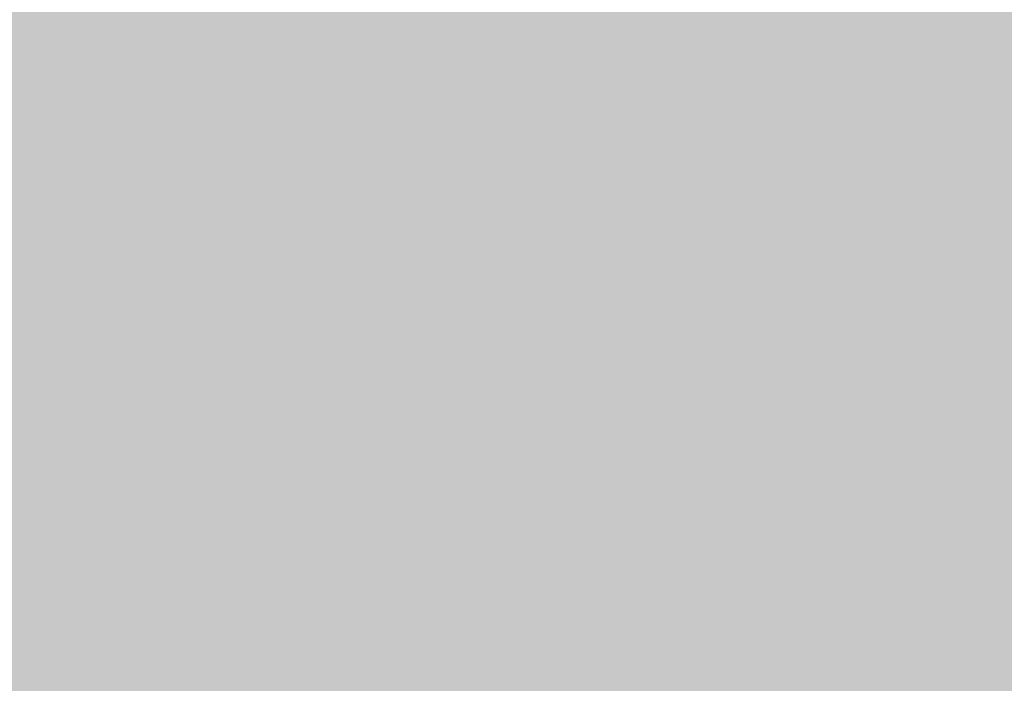
# Model space of a CAD drawing. Units: feet. Extents: x 3168 to 4724, y 827 to 1477.
# Tile 140 of 256: x 3301.134076 to 3301.1362, y 1099.01485 to 1099.016281. Entities that reach past the tile are written whole.
import ezdxf

# ---------------------------------------------------------------- set-up
doc = ezdxf.new("R2010")
doc.units = ezdxf.units.FT
doc.layers.add('A-ELEV', color=7, linetype='Continuous', lineweight=35)
doc.layers.add('A-ELEV-PATT', color=8, linetype='Continuous', lineweight=13)

msp = doc.modelspace()

# ---------------------------------------------------------------- hatches: boundary and pattern name
at = {"layer": 'A-ELEV-PATT'}
h = msp.add_hatch(color=256, dxfattribs=at)
h.dxf.hatch_style = 1
edge = h.paths.add_edge_path()
edge.add_ellipse((3552.9057615, 979.2201412), major_axis=(36.7449243, 0), ratio=0.4848484848, start_angle=0, end_angle=360)
edge = h.paths.add_edge_path()
edge.add_ellipse((3559.8916366, 929.2522824), major_axis=(36.7449243, 0), ratio=0.4848484848, start_angle=0, end_angle=360)
edge = h.paths.add_edge_path()
edge.add_line((3299.3168105, 1198.606081), (3479.9167135, 1198.606081))
edge.add_line((3479.9167135, 1198.606081), (3479.9167135, 1209.8685704))
edge.add_spline(control_points=[(3479.9167135, 1209.8685704), (3464.3011571, 1209.8685704), (3448.6856007, 1209.8685704), (3410.949139, 1209.8685704), (3388.8282339, 1209.8685704), (3355.6468761, 1209.8685704), (3344.5864235, 1209.8685704), (3327.9957446, 1209.8685704), (3322.4655183, 1209.8685704), (3314.1701788, 1209.8685704), (3311.4050657, 1209.8685704), (3307.257396, 1209.8685704), (3305.8748394, 1209.8685704), (3303.8010045, 1209.8685704), (3303.1097262, 1209.8685704), (3302.0728088, 1209.8685704), (3301.7271697, 1209.8685704), (3301.2087109, 1209.8685704), (3301.0358914, 1209.8685704), (3300.776662, 1209.8685704), (3300.6902522, 1209.8685704), (3300.5606376, 1209.8685704), (3300.5174327, 1209.8685704), (3300.4526253, 1209.8685704), (3300.4310229, 1209.8685704), (3300.3986192, 1209.8685704), (3300.387818, 1209.8685704), (3300.3662155, 1209.8685704), (3300.3456757, 1209.8685704), (3300.3455476, 1209.8685704), (3300.345505, 1209.8685704), (3300.3433041, 1209.8685704), (3300.341146, 1209.8685707), (3300.337909, 1209.8685714), (3300.33683, 1209.8685718), (3300.3339422, 1209.8685728), (3300.3321334, 1209.8685736), (3300.3255154, 1209.8685773), (3300.3207065, 1209.8685812), (3300.3109248, 1209.8685917), (3300.305952, 1209.8685984), (3300.2905113, 1209.8686233), (3300.2800452, 1209.8686461), (3300.2324255, 1209.868777), (3300.1952979, 1209.868954), (3299.9510684, 1209.8706077), (3299.7448244, 1209.8743259), (3299.4368271, 1209.8832566), (3299.3343894, 1209.8867924), (3299.181079, 1209.8929197), (3299.1300333, 1209.8950994), (3298.6522171, 1209.9168011), (3298.2294605, 1209.9457176), (3297.6016312, 1210.0023671), (3297.3934043, 1210.0234637), (3297.082652, 1210.058309), (3296.9793324, 1210.0704575), (3296.2929541, 1210.1548606), (3295.7181475, 1210.2433556), (3294.8687167, 1210.3988504), (3294.5876997, 1210.4544779), (3294.1693407, 1210.5433488), (3294.0304153, 1210.5738777), (3291.7071487, 1211.1012), (3289.6535901, 1211.8134353), (3285.7762586, 1213.5639876), (3283.9514101, 1214.6034778), (3280.512159, 1216.9800798), (3278.8972407, 1218.3175918), (3276.3799143, 1220.829489), (3275.4160415, 1221.9177379), (3274.0393421, 1223.7076996), (3273.5810428, 1224.3495346), (3273.1432283, 1225.0163162)], knot_values=[39.119033, 39.119033, 39.119033, 39.119033, 39.286353, 39.286353, 39.523379, 39.523379, 39.641892, 39.641892, 39.701148, 39.701148, 39.730777, 39.730777, 39.745591, 39.745591, 39.752998, 39.752998, 39.756701, 39.756701, 39.758553, 39.758553, 39.759479, 39.759479, 39.759942, 39.759942, 39.760173, 39.760173, 39.760289, 39.760289, 39.760405, 39.760405, 39.760463, 39.760463, 39.763389, 39.763389, 39.764851, 39.764851, 39.767304, 39.767304, 39.773825, 39.773825, 39.78057, 39.78057, 39.79477, 39.79477, 39.845194, 39.845194, 40.126715, 40.126715, 40.267476, 40.267476, 40.337856, 40.337856, 40.927023, 40.927023, 41.221606, 41.221606, 41.368898, 41.368898, 42.202622, 42.202622, 42.619485, 42.619485, 42.827916, 42.827916, 46.118323, 46.118323, 49.408731, 49.408731, 52.699139, 52.699139, 54.927489, 54.927489, 56.104228, 56.104228, 56.104228, 56.104228], weights=[1, 1, 1, 1, 1, 1, 1, 1, 1, 1, 1, 1, 1, 1, 1, 1, 1, 1, 1, 1, 1, 1, 1, 1, 1, 1, 1, 1, 1, 1, 1, 1, 1, 1, 1, 1, 1, 1, 1, 1, 1, 1, 1, 1, 1, 1, 1, 1, 1, 1, 1, 1, 1, 1, 1, 1, 1, 1, 1, 1, 1, 1, 1, 1, 1, 1, 1, 1, 1, 1, 1, 1, 1, 1], degree=3, periodic=0)
edge.add_line((3273.1432283, 1225.0163162), (3273.1432283, 1099.0163162))
edge.add_line((3273.1432283, 1099.0163162), (3299.3168105, 1099.0163162))
edge.add_line((3299.3168105, 1099.0163162), (3299.3168105, 1198.606081))
edge = h.paths.add_edge_path()
edge.add_line((3304.7584434, 1324.15806), (3479.9167135, 1324.15806))
edge.add_line((3479.9167135, 1324.15806), (3479.9167135, 1335.7146184))
edge.add_line((3479.9167135, 1335.7146184), (3269.1616284, 1335.7146184))
edge.add_spline(control_points=[(3269.1616284, 1335.7146184), (3264.0242315, 1335.7146184), (3258.364118, 1328.9581888), (3259.2643109, 1323.9002743)], knot_values=[0, 0, 0, 0, 15.412191, 15.412191, 15.412191, 15.412191], degree=3, periodic=0)
edge.add_line((3259.2643109, 1323.9002743), (3265.5168487, 1288.7691348))
edge.add_line((3265.5168487, 1288.7691348), (3275.2651026, 1261.5456259))
edge.add_line((3275.2651026, 1261.5456259), (3304.7584434, 1261.5456259))
edge.add_line((3304.7584434, 1261.5456259), (3304.7584434, 1324.15806))
h = msp.add_hatch(color=256, dxfattribs=at)
h.dxf.hatch_style = 1
h.paths.add_polyline_path([(3384.5252473, 1099.0163162), (3335.0291678, 1099.0163162), (3299.3168105, 1099.0163162), (3273.1432283, 1099.0163162), (3217.5653642, 1099.0163162), (3168.0692847, 827.1162598), (3335.0291678, 827.1162598)])

# ---------------------------------------------------------------- linework, layer by layer
at = {"layer": 'A-ELEV'}
msp.add_open_spline([(3808.5202001, 1099.0163162), (3808.5202001, 1141.413235), (3808.5202001, 1183.8101539), (3808.5202001, 1226.6353244), (3808.5202001, 1227.0635761), (3808.5202001, 1227.4918279), (3811.491871, 1248.9946729), (3814.463542, 1270.497518), (3817.4652299, 1292.2175635), (3817.4952467, 1292.434764), (3817.5252636, 1292.6519644), (3817.5728014, 1310.1067483), (3817.6203393, 1327.5615322), (3817.6678771, 1345.0163162), (3817.6678771, 1345.4579619), (3817.6678771, 1345.8996077), (3817.6678771, 1346.4560466), (3817.6678771, 1346.5708398), (3817.6678771, 1346.7528874), (3817.6678771, 1346.8201418), (3817.6678771, 1346.9348705), (3817.6678771, 1346.9823447), (3817.6678771, 1347.0385872), (3817.6678771, 1347.0473556), (3817.6678771, 1347.0736607), (3817.667877, 1347.0593025), (3817.6678766, 1347.0615455), (3817.6678764, 1347.0626669), (3817.6678754, 1347.0660311), (3817.6678743, 1347.0682738), (3817.6678701, 1347.0750012), (3817.667866, 1347.0794856), (3817.6678493, 1347.0929368), (3817.6678325, 1347.1019019), (3817.6677657, 1347.1287896), (3817.6676988, 1347.1467049), (3817.6674317, 1347.2004211), (3817.6671649, 1347.2361922), (3817.6661003, 1347.3433849), (3817.6650383, 1347.4146859), (3817.6608124, 1347.6280949), (3817.6566084, 1347.7697085), (3817.6399698, 1348.1924868), (3817.6235091, 1348.4715855), (3817.5590944, 1349.3000666), (3817.4961208, 1349.8405878), (3817.2554319, 1351.4241561), (3817.0263177, 1352.4287852), (3816.3068713, 1354.8889138), (3815.7437452, 1356.2687272), (3814.4639586, 1358.8192105), (3813.7464132, 1359.9909676), (3812.1958378, 1362.1723433), (3811.3622453, 1363.1821237), (3809.5888357, 1365.0690087), (3808.6488164, 1365.9461052), (3806.6542623, 1367.5796162), (3805.5997024, 1368.336154), (3803.3528906, 1369.7223272), (3802.1605354, 1370.352386), (3799.6008131, 1371.4535864), (3798.2326878, 1371.9254812), (3795.2800838, 1372.6346239), (3793.6931479, 1372.8720685), (3791.8694413, 1372.9264797), (3791.7408615, 1372.9292203), (3791.3533713, 1372.9341014), (3791.0927074, 1372.9329013), (3790.3041163, 1372.9150676), (3789.7695426, 1372.8841946), (3789.20919, 1372.8302363), (3789.1906217, 1372.8284241), (3789.1348916, 1372.8229123), (3789.097705, 1372.8191375), (3789.0484446, 1372.8140077), (3789.0364001, 1372.8127432), (3789.0002562, 1372.808918), (3788.9761468, 1372.8063255), (3788.9494049, 1372.8034042), (3788.9467858, 1372.8031177), (3788.9425667, 1372.8026552), (3788.9409669, 1372.8024797), (3788.9385718, 1372.8022166), (3788.9377765, 1372.8021292), (3788.9353908, 1372.8018669), (3788.8675349, 1372.7944024), (3788.7568665, 1372.7822285), (3788.7015323, 1372.7761415), (3788.5355297, 1372.7578805), (3788.4248612, 1372.7457065), (3788.092856, 1372.7091846), (3787.8715192, 1372.6848366), (3787.2075086, 1372.6117927), (3786.764835, 1372.5630968), (3785.436814, 1372.417009), (3784.5514666, 1372.3196171), (3781.8954246, 1372.0274416), (3780.1247299, 1371.8326579), (3774.8126458, 1371.2483067), (3771.2712564, 1370.8587393), (3760.6470883, 1369.6900371), (3753.5643095, 1368.9109022), (3732.3159732, 1366.5734977), (3718.1504157, 1365.015228), (3694.0067577, 1362.3593262), (3684.0286573, 1361.2616941), (3674.0505568, 1360.1640619), (3664.6006617, 1360.1640619), (3655.1507666, 1360.1640619), (3626.8010812, 1360.1640619), (3607.9012909, 1360.1640619), (3551.2019201, 1360.1640619), (3513.4023395, 1360.1640619), (3467.7251817, 1360.1640619), (3459.8476045, 1360.1640619), (3436.2148727, 1360.1640619), (3420.4597182, 1360.1640619), (3373.1942547, 1360.1640619), (3341.6839457, 1360.1640619), (3302.8481616, 1360.1640619), (3295.5226865, 1360.1640619), (3286.0382916, 1360.1640619), (3283.8793719, 1360.1640619), (3277.4026128, 1360.1640619), (3273.0847733, 1360.1640619), (3267.7328511, 1360.1640619), (3266.6987684, 1360.1640619), (3263.5965201, 1360.1640619), (3261.5283546, 1360.1640619), (3259.2369429, 1360.1640619), (3259.0136967, 1360.1640619), (3258.3439582, 1360.1640619), (3257.8974658, 1360.1640619), (3257.4309979, 1360.1640619), (3257.4110224, 1360.1640619), (3257.3705735, 1360.1640619), (3257.3754695, 1360.1640619), (3257.3745975, 1360.1640619), (3257.3739371, 1360.1640618), (3257.3719559, 1360.1640616), (3257.3706351, 1360.1640613), (3257.366673, 1360.16406), (3257.3640318, 1360.1640586), (3257.3561088, 1360.1640529), (3257.3508277, 1360.1640469), (3257.3349869, 1360.1640226), (3257.3244299, 1360.163998), (3257.2927692, 1360.1638987), (3257.2716761, 1360.1637987), (3257.208439, 1360.1633975), (3257.1663373, 1360.1629953), (3257.0402058, 1360.1613882), (3256.9563493, 1360.1597827), (3256.705504, 1360.1533932), (3256.53924, 1360.1470361), (3256.0435702, 1360.1219156), (3255.717296, 1360.0971018), (3254.7524458, 1360.0004808), (3254.1279679, 1359.906513), (3252.1800666, 1359.5253322), (3250.9415739, 1359.1439911), (3248.6701751, 1358.2432905), (3247.6357388, 1357.7238339), (3245.7326321, 1356.6034712), (3244.8633884, 1356.0020595), (3243.2531076, 1354.7428655), (3242.511972, 1354.0847309), (3240.7510518, 1352.3447812), (3239.8009609, 1351.229574), (3238.0877694, 1348.8724402), (3237.3246853, 1347.6303552), (3235.9825098, 1344.9716321), (3235.4022051, 1343.554907), (3234.5910812, 1340.8154577), (3234.3108819, 1339.5435498), (3233.9764902, 1336.8025605), (3233.9221126, 1335.3308771), (3234.1489156, 1332.5912693), (3234.3495287, 1331.3672011), (3234.7198926, 1329.9993668), (3234.7524228, 1329.8833616), (3234.853619, 1329.5347966), (3234.9258923, 1329.301685), (3235.0248359, 1329.0025524), (3235.0469235, 1328.936928), (3235.0776388, 1328.8472393), (3235.0859239, 1328.8231979), (3235.1109389, 1328.7510642), (3235.1278282, 1328.7029624), (3235.1479919, 1328.6462418), (3235.1510592, 1328.6376324), (3235.1560959, 1328.6235265), (3235.1580611, 1328.6180301), (3235.1602094, 1328.6120302), (3235.1656119, 1328.596943), (3235.1800989, 1328.556486), (3235.190263, 1328.5281009), (3235.2207556, 1328.4429457), (3235.241084, 1328.3861755), (3235.3020692, 1328.215865), (3235.3427259, 1328.1023247), (3235.4646962, 1327.7617038), (3235.5460097, 1327.5346232), (3235.7899503, 1326.8533813), (3235.9525774, 1326.39922), (3236.4404586, 1325.0367362), (3236.7657127, 1324.1284137), (3237.7414751, 1321.4034462), (3238.3919833, 1319.5868011), (3240.3435081, 1314.136866), (3241.6445245, 1310.503576), (3245.547574, 1299.6037058), (3248.149607, 1292.3371257), (3255.955706, 1270.5373853), (3261.1597719, 1256.004225), (3267.3876177, 1238.6120011), (3268.4113975, 1235.7529374), (3269.5103781, 1232.6838639), (3269.5855789, 1232.473854), (3269.7066118, 1232.1358507), (3269.752444, 1232.0078573), (3269.8273289, 1231.7987296), (3269.8563817, 1231.7175953), (3269.9063247, 1231.5781217), (3269.927215, 1231.5197823), (3269.9724682, 1231.3934057), (3269.9968311, 1231.3253685), (3270.0265026, 1231.2425062), (3270.0318112, 1231.2276812), (3270.0402823, 1231.2040243), (3270.0392242, 1231.2069792), (3270.0393595, 1231.2066014), (3270.0394271, 1231.2064125), (3270.0396301, 1231.2058458), (3270.0397654, 1231.205468), (3270.0401713, 1231.2043346), (3270.040442, 1231.2035791), (3270.041254, 1231.2013125), (3270.0417955, 1231.1998016), (3270.0434203, 1231.195269), (3270.044504, 1231.1922477), (3270.0477563, 1231.1831849), (3270.0499263, 1231.1771446), (3270.0564418, 1231.1590283), (3270.0607927, 1231.146957), (3270.0738674, 1231.1107614), (3270.0826128, 1231.0866558), (3270.1089357, 1231.0144129), (3270.1265997, 1230.9663498), (3270.1799341, 1230.8224568), (3270.2159467, 1230.7269233), (3270.3253234, 1230.4415078), (3270.4000257, 1230.2528107), (3270.6292491, 1229.6914436), (3270.7888829, 1229.3235005), (3271.2864875, 1228.2383194), (3271.6430996, 1227.5397546), (3272.7758592, 1225.515277), (3273.6141694, 1224.2605021), (3275.4160415, 1221.9177379), (3276.3799143, 1220.829489), (3278.8972407, 1218.3175918), (3280.512159, 1216.9800798), (3283.9514101, 1214.6034778), (3285.7762586, 1213.5639876), (3289.6535901, 1211.8134353), (3291.7071487, 1211.1012), (3294.0304153, 1210.5738777), (3294.1693407, 1210.5433488), (3294.5876997, 1210.4544779), (3294.8687167, 1210.3988504), (3295.7181475, 1210.2433556), (3296.2929541, 1210.1548606), (3296.9793324, 1210.0704575), (3297.082652, 1210.058309), (3297.3934043, 1210.0234637), (3297.6016312, 1210.0023671), (3298.2294605, 1209.9457176), (3298.6522171, 1209.9168011), (3299.1300333, 1209.8950994), (3299.181079, 1209.8929197), (3299.3343894, 1209.8867924), (3299.4368271, 1209.8832566), (3299.7448244, 1209.8743259), (3299.9510684, 1209.8706077), (3300.1952979, 1209.868954), (3300.2324255, 1209.868777), (3300.2800452, 1209.8686461), (3300.2905113, 1209.8686233), (3300.305952, 1209.8685984), (3300.3109248, 1209.8685917), (3300.3207065, 1209.8685812), (3300.3255154, 1209.8685773), (3300.3321334, 1209.8685736), (3300.3339422, 1209.8685728), (3300.33683, 1209.8685718), (3300.337909, 1209.8685714), (3300.341146, 1209.8685707), (3300.3433041, 1209.8685704), (3300.345505, 1209.8685704), (3300.3455476, 1209.8685704), (3300.3456757, 1209.8685704), (3300.3662155, 1209.8685704), (3300.387818, 1209.8685704), (3300.3986192, 1209.8685704), (3300.4310229, 1209.8685704), (3300.4526253, 1209.8685704), (3300.5174327, 1209.8685704), (3300.5606376, 1209.8685704), (3300.6902522, 1209.8685704), (3300.776662, 1209.8685704), (3301.0358914, 1209.8685704), (3301.2087109, 1209.8685704), (3301.7271697, 1209.8685704), (3302.0728088, 1209.8685704), (3303.1097262, 1209.8685704), (3303.8010045, 1209.8685704), (3305.8748394, 1209.8685704), (3307.257396, 1209.8685704), (3311.4050657, 1209.8685704), (3314.1701788, 1209.8685704), (3322.4655183, 1209.8685704), (3327.9957446, 1209.8685704), (3344.5864235, 1209.8685704), (3355.6468761, 1209.8685704), (3388.8282339, 1209.8685704), (3410.949139, 1209.8685704), (3477.3118546, 1209.8685704), (3521.553665, 1209.8685704), (3566.8361836, 1209.8685704), (3567.8768919, 1209.8685704), (3570.9990167, 1209.8685704), (3573.0804332, 1209.8685704), (3575.7813964, 1209.8685704), (3576.4009432, 1209.8685704), (3577.2958211, 1209.8685704), (3577.5711523, 1209.8685704), (3578.3971458, 1209.8685704), (3578.9478081, 1209.8685704), (3579.7564907, 1209.8685704), (3580.0145108, 1209.8685704), (3580.3427367, 1209.8685704), (3580.3268649, 1209.8685704), (3580.3271702, 1209.8685704), (3580.3273229, 1209.8685704), (3580.3277809, 1209.8685704), (3580.3280863, 1209.8685704), (3580.3290024, 1209.8685703), (3580.3296132, 1209.8685702), (3580.3314455, 1209.8685699), (3580.332667, 1209.8685697), (3580.336332, 1209.8685685), (3580.3387755, 1209.8685674), (3580.3461066, 1209.8685629), (3580.350995, 1209.8685584), (3580.3656627, 1209.8685402), (3580.3754446, 1209.868522), (3580.4048012, 1209.8684493), (3580.4243863, 1209.8683764), (3580.4831833, 1209.8680848), (3580.5224371, 1209.8677929), (3580.6403612, 1209.8666242), (3580.7191947, 1209.8654543), (3580.9563152, 1209.8607663), (3581.1152222, 1209.85607), (3581.5941635, 1209.8372298), (3581.9164188, 1209.8183314), (3582.8899466, 1209.7424284), (3583.547986, 1209.6661692), (3585.5318268, 1209.3606172), (3586.8672159, 1209.0538859), (3589.4715454, 1208.2524717), (3590.7402412, 1207.7578521), (3591.9954511, 1207.1588024), (3592.057809, 1207.1287398), (3592.2442418, 1207.0379536), (3592.3676757, 1206.9766317), (3592.73528, 1206.7903591), (3592.9767518, 1206.663101), (3593.2445387, 1206.5164414), (3593.2747313, 1206.4998248), (3593.3651153, 1206.4498388), (3593.4251129, 1206.4163333), (3593.6043138, 1206.3152851), (3593.7227254, 1206.2472105), (3593.8572122, 1206.1683978), (3593.8743621, 1206.1583193), (3593.925741, 1206.1280407), (3593.9598989, 1206.1077976), (3594.0620855, 1206.0468991), (3594.1298272, 1206.0060745), (3594.2084359, 1205.9581709), (3594.2196829, 1205.9513043), (3594.253391, 1205.9306863), (3594.2758193, 1205.9169166), (3594.3429716, 1205.8755358), (3594.3875633, 1205.8478526), (3594.4336161, 1205.8190499), (3594.4352559, 1205.818024), (3594.4401746, 1205.8149461), (3594.4434527, 1205.8128936), (3594.4471229, 1205.8105944), (3594.4475159, 1205.8103482), (3594.4486949, 1205.8096095), (3594.4494808, 1205.8091171), (3594.4503663, 1205.8085621), (3594.4504658, 1205.8084998), (3594.4506003, 1205.8084155), (3594.4673993, 1205.7978872), (3594.4932689, 1205.7816741), (3594.5062037, 1205.7735675), (3594.5450081, 1205.7492479), (3594.5708778, 1205.7330348), (3594.6484866, 1205.6843956), (3594.7002258, 1205.6519694), (3594.8554436, 1205.5546909), (3594.958922, 1205.4898386), (3595.2693574, 1205.2952816), (3595.4763144, 1205.1655769), (3596.0971852, 1204.7764629), (3596.5110991, 1204.5170536), (3597.7528407, 1203.7388256), (3598.5806685, 1203.220007), (3601.0641518, 1201.663551), (3602.7198073, 1200.6259137), (3607.686774, 1197.5130018), (3610.998085, 1195.4377272), (3620.9320182, 1189.2119034), (3627.5546404, 1185.0613542), (3647.4225068, 1172.6097066), (3660.6677511, 1164.3086082), (3700.403484, 1139.405313), (3726.8939725, 1122.8031161), (3757.2057154, 1103.8060516), (3761.0269697, 1101.4111839), (3764.848224, 1099.0163162), (3745.3282713, 1099.0163162), (3725.8083186, 1099.0163162), (3706.288366, 1099.0163162), (3706.288366, 1108.4532371), (3706.288366, 1117.890158), (3706.288366, 1127.3270789), (3710.7507544, 1127.3270789), (3715.2131428, 1127.3270789), (3719.6755312, 1127.3270789)], degree=3, knots=[0, 0, 0, 0, 0.982037, 0.982037, 0.991957, 0.991957, 0.991957, 1.966522, 1.966522, 1.976367, 1.976367, 1.976367, 2.976367, 2.976367, 2.976367, 3.00169, 3.00169, 3.008272, 3.008272, 3.012129, 3.012129, 3.014851, 3.014851, 3.015353, 3.015353, 3.016359, 3.016359, 3.017365, 3.017365, 3.019376, 3.019376, 3.023398, 3.023398, 3.031442, 3.031442, 3.047531, 3.047531, 3.079708, 3.079708, 3.144063, 3.144063, 3.272772, 3.272772, 3.53019, 3.53019, 4.045026, 4.045026, 5.074698, 5.074698, 6.700878, 6.700878, 8.327058, 8.327058, 9.953238, 9.953238, 11.579418, 11.579418, 13.205598, 13.205598, 14.831778, 14.831778, 16.457958, 16.457958, 18.084138, 18.084138, 18.206872, 18.206872, 18.45234, 18.45234, 18.943275, 18.943275, 18.960093, 18.960093, 18.993729, 18.993729, 19.00461, 19.00461, 19.026374, 19.026374, 19.028737, 19.028737, 19.03018, 19.03018, 19.030897, 19.030897, 19.032332, 19.032332, 19.033766, 19.033766, 19.036636, 19.036636, 19.042374, 19.042374, 19.053851, 19.053851, 19.076805, 19.076805, 19.122714, 19.122714, 19.21453, 19.21453, 19.398163, 19.398163, 19.765429, 19.765429, 20.024128, 20.024128, 20.024128, 20.092031, 20.092031, 20.227836, 20.227836, 20.499446, 20.499446, 20.556051, 20.556051, 20.66926, 20.66926, 20.895678, 20.895678, 20.948316, 20.948316, 20.963829, 20.963829, 20.994855, 20.994855, 21.002285, 21.002285, 21.017146, 21.017146, 21.01875, 21.01875, 21.021959, 21.021959, 21.022102, 21.022102, 21.022249, 21.022249, 21.022708, 21.022708, 21.023627, 21.023627, 21.025464, 21.025464, 21.029138, 21.029138, 21.036486, 21.036486, 21.051183, 21.051183, 21.080575, 21.080575, 21.139361, 21.139361, 21.256932, 21.256932, 21.492073, 21.492073, 21.962356, 21.962356, 23.01002, 23.01002, 24.057684, 24.057684, 25.105348, 25.105348, 26.153011, 26.153011, 27.776787, 27.776787, 29.400562, 29.400562, 31.024337, 31.024337, 32.278801, 32.278801, 33.533265, 33.533265, 34.467568, 34.467568, 34.553971, 34.553971, 34.726776, 34.726776, 34.775309, 34.775309, 34.793079, 34.793079, 34.82862, 34.82862, 34.834979, 34.834979, 34.839039, 34.839039, 34.839411, 34.839411, 34.840285, 34.840285, 34.842034, 34.842034, 34.845531, 34.845531, 34.852525, 34.852525, 34.866512, 34.866512, 34.894488, 34.894488, 34.950439, 34.950439, 35.062342, 35.062342, 35.286147, 35.286147, 35.733758, 35.733758, 35.821815, 35.821815, 35.828283, 35.828283, 35.832225, 35.832225, 35.834724, 35.834724, 35.836521, 35.836521, 35.838617, 35.838617, 35.839073, 35.839073, 35.839345, 35.839345, 35.839617, 35.839617, 35.840161, 35.840161, 35.841249, 35.841249, 35.843425, 35.843425, 35.847778, 35.847778, 35.856482, 35.856482, 35.873891, 35.873891, 35.908709, 35.908709, 35.978345, 35.978345, 36.117617, 36.117617, 36.396161, 36.396161, 36.953248, 36.953248, 38.067423, 38.067423, 40.295772, 40.295772, 42.524122, 42.524122, 45.81453, 45.81453, 49.104937, 49.104937, 52.395345, 52.395345, 52.603776, 52.603776, 53.020639, 53.020639, 53.854363, 53.854363, 54.001655, 54.001655, 54.296238, 54.296238, 54.885405, 54.885405, 54.955785, 54.955785, 55.096546, 55.096546, 55.378067, 55.378067, 55.42849, 55.42849, 55.442691, 55.442691, 55.449436, 55.449436, 55.455957, 55.455957, 55.458409, 55.458409, 55.459872, 55.459872, 55.462798, 55.462798, 55.462856, 55.462856, 55.462972, 55.462972, 55.463088, 55.463088, 55.463319, 55.463319, 55.463782, 55.463782, 55.464708, 55.464708, 55.46656, 55.46656, 55.470263, 55.470263, 55.47767, 55.47767, 55.492484, 55.492484, 55.522112, 55.522112, 55.581369, 55.581369, 55.699882, 55.699882, 55.936907, 55.936907, 56.410959, 56.410959, 56.42211, 56.42211, 56.444413, 56.444413, 56.451051, 56.451051, 56.454001, 56.454001, 56.459901, 56.459901, 56.462666, 56.462666, 56.463418, 56.463418, 56.464171, 56.464171, 56.465675, 56.465675, 56.468684, 56.468684, 56.474702, 56.474702, 56.486738, 56.486738, 56.51081, 56.51081, 56.558955, 56.558955, 56.655243, 56.655243, 56.847821, 56.847821, 57.232975, 57.232975, 58.003284, 58.003284, 59.543901, 59.543901, 62.625137, 62.625137, 68.787607, 68.787607, 74.950078, 74.950078, 75.27336, 75.27336, 75.919923, 75.919923, 77.213051, 77.213051, 77.377769, 77.377769, 77.707206, 77.707206, 78.366079, 78.366079, 78.462532, 78.462532, 78.655436, 78.655436, 79.041245, 79.041245, 79.105735, 79.105735, 79.234714, 79.234714, 79.492672, 79.492672, 79.502197, 79.502197, 79.521249, 79.521249, 79.523534, 79.523534, 79.528103, 79.528103, 79.528682, 79.528682, 79.528885, 79.528885, 79.529089, 79.529089, 79.529495, 79.529495, 79.530308, 79.530308, 79.531935, 79.531935, 79.535187, 79.535187, 79.541693, 79.541693, 79.554704, 79.554704, 79.580725, 79.580725, 79.632769, 79.632769, 79.736856, 79.736856, 79.94503, 79.94503, 80.361377, 80.361377, 80.421435, 80.421435, 80.421435, 81.421435, 81.421435, 81.421435, 82.421435, 82.421435, 82.421435, 83.421435, 83.421435, 83.421435, 83.421435], dxfattribs=at)

doc.saveas('drawing.dxf')
